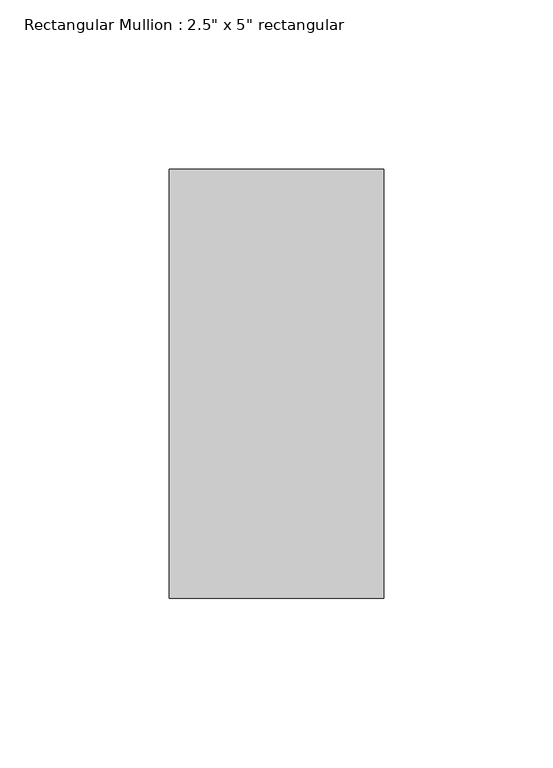
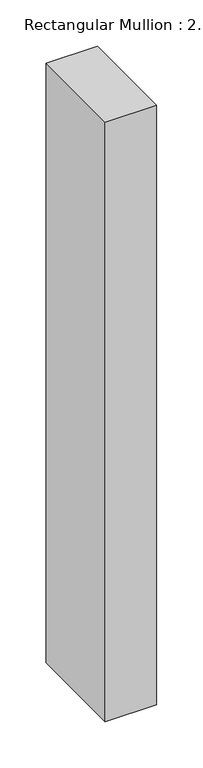
"""IFC4 building model written with IfcOpenShell, lengths in millimetres: member geometry."""

from ifc_helpers import new_model, si_unit, frame, origin, place, context, project, spatial, polyline, outline, extrude, source, transform, mapped, element, save


def member_18a184ad(model_context):
    return source(origin(), model_context, "Body", "SweptSolid", [
        extrude(outline(polyline([(31.75, 63.5), (31.75, -63.5), (-31.75, -63.5), (-31.75, 63.5), (31.75, 63.5)])), frame((0.0, 0.0, -787.4), z_axis=(0.0, 0.0, 1.0), x_axis=(1.0, 0.0, 0.0)), (0.0, 0.0, 1.0), 787.4),
    ])


if __name__ == "__main__":
    model = new_model("IFC4")
    model_context = context("Model", 3, world=origin())
    ifc_project = project(units=[si_unit("LENGTHUNIT", "METRE", prefix="MILLI")], contexts=[model_context])
    site = spatial("IfcSite", under=ifc_project)
    building = spatial("IfcBuilding", under=site)
    placement = place(None, origin())
    member_shape = member_18a184ad(model_context)
    element("IfcMember", 1, ObjectType="Rectangular Mullion : 2.5\" x 5\" rectangular", at=placement, inside=building, context=model_context, shape_type="MappedRepresentation", body=[
        mapped(member_shape, transform((0.0, 0.0, 0.0), x_axis=(1.0, 0.0, 0.0), y_axis=(0.0, 1.0, 0.0), z_axis=(0.0, 0.0, 1.0))),
    ])
    save(model, "model.ifc")

# Revit data of these elements
# Type "Rectangular Mullion : 2.5\" x 5\" rectangular"
#   built-in parameter 1007304 = 0.416667 (stored number, unit not read)
#   built-in parameter 1007301 = 0.104167 (stored number, unit not read)
#   built-in parameter 1007300 = 0.104167 (stored number, unit not read)
# Element 1 (IfcMember, "Rectangular Mullion : 2.5\" x 5\" rectangular")
#   Materials on its faces: "Aluminum"
# Materials
#   "Aluminum": class "Metal", colour RGB 247 247 247, transparency 0, Description = "Aluminum 6061", Cost = 0
